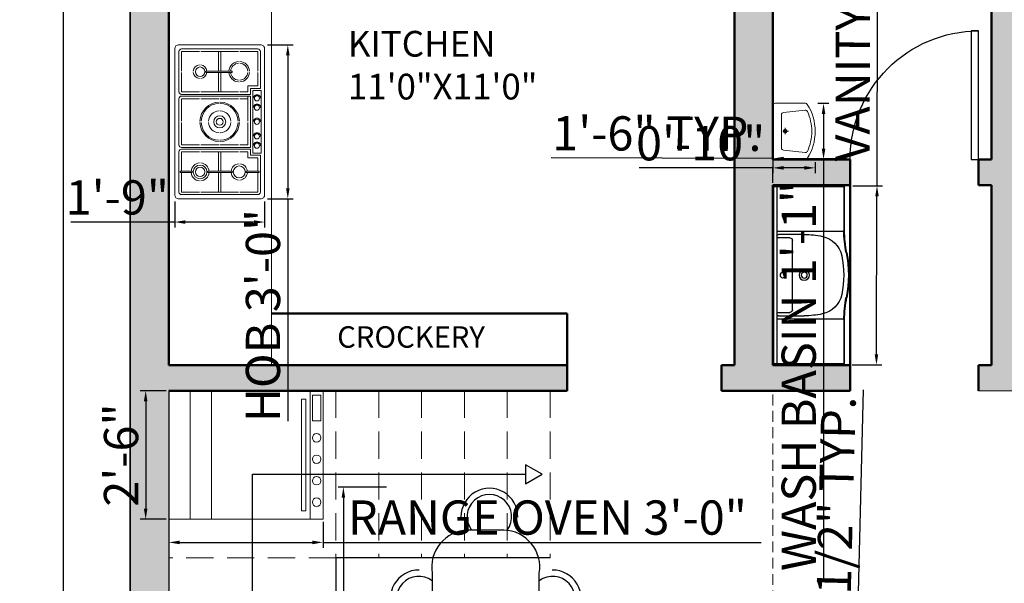
# Model space of a CAD drawing. Units: inches. Extents: x 3354 to 4308, y 1668 to 2317.
# Tile 6 of 11: x 3370 to 3600, y 2066 to 2198. Entities that reach past the tile are written whole.
import ezdxf

# ---------------------------------------------------------------- set-up
doc = ezdxf.new("R2010")
doc.units = ezdxf.units.IN
doc.linetypes.add('DASHED', pattern=[19.05, 12.7, -6.35])
for name, color, linetype, lineweight in [('A-ANNO-DIMS', 2, 'Continuous', 18), ('A-ANNO-TEXT', 7, 'Continuous', 18), ('A-AREA-IDEN', 3, 'Continuous', 18), ('A-DOOR', 3, 'Continuous', 25), ('A-EQPM', 9, 'Continuous', 18), ('A-FLOR-FIXT', 8, 'Continuous', 18), ('A-FLOR-OVHD', 8, 'DASHED', 18), ('A-FLOR-STRS', 7, 'Continuous', 25), ('A-FURN', 8, 'Continuous', 18), ('A-GLAZ', 4, 'Continuous', 18), ('A-WALL', 7, 'Continuous', 50), ('A-WALL-PATT', 8, 'Continuous', 13), ('C-PROP', 1, 'Continuous', 35)]:
    doc.layers.add(name, color=color, linetype=linetype, lineweight=lineweight)
doc.layers.add('furniture', color=7, linetype='Continuous')
doc.layers.add('SANTEH', color=7, linetype='Continuous')
doc.styles.get("Standard").update_dxf_attribs({"font": 'arial.ttf'})
doc.dimstyles.new('ISO-25', dxfattribs={"dimtxt": 8, "dimasz": 2.5, "dimexe": 1.25, "dimexo": 0.625, "dimtad": 1, "dimdec": 1, "dimlunit": 3, "dimtxsty": 'Standard', "dimcen": 2.5, "dimadec": 0, "dimazin": 0, "dimtfac": 1, "dimtdec": 1, "dimtmove": 0, "dimatfit": 3, "dimfxl": 1, "dimarcsym": 0})

# ---------------------------------------------------------------- blocks, each defined once
blk = doc.blocks.new('*U2')
for p, q in [((0, 0), (0, -6)), ((30, 0), (30, -6))]:
    blk.add_line(p, q)
blk.add_lwpolyline([(0, 0), (0, 30), (1.75, 30), (1.75, 0)], close=True)
blk.add_arc((0, 0), 30, 0, 90)
blk = doc.blocks.new('STOVE')
for p, q in [((11.85, 19.7), (11.55, 19.7)), ((11.55, 16.92), (11.55, 19.7)), ((11.85, 16.92), (11.85, 19.7)), ((11.85, 16.92), (11.55, 16.92)), ((-11.85, 13.73), (-11.85, 7.62)), ((-11.85, 13.73), (-11.55, 13.73)), ((-11.55, 13.73), (-11.55, 7.62)), ((11.85, 13.23), (11.55, 13.23)), ((11.55, 13.23), (11.55, 7.57)), ((11.85, 13.23), (11.85, 7.57)), ((-11.85, 10.75), (-16.4, 10.75)), ((-11.85, 10.25), (-16.4, 10.25)), ((-7, 10.75), (-11.55, 10.75)), ((-7, 10.25), (-11.55, 10.25)), ((7, 10.75), (11.55, 10.75)), ((7, 10.25), (11.55, 10.25)), ((11.85, 10.75), (16.4, 10.75)), ((11.85, 10.25), (16.4, 10.25)), ((-11.85, 7.62), (-11.55, 7.62)), ((11.85, 7.57), (11.55, 7.57)), ((-7, 3.9), (-8.4, 3.9)), ((-7.8, 3.3), (-7.8, 1)), ((-6.4, 3.3), (-7.8, 3.3)), ((7.3, 2.8), (-7.3, 2.8)), ((-7.3, 2.8), (-7.3, 0.8)), ((-5.4, 3.9), (-6, 3.9)), ((-5.4, 3.9), (-0.15, 3.9)), ((0.15, 3.9), (5.4, 3.9)), ((6.4, 3.3), (7.8, 3.3)), ((7, 3.9), (8.4, 3.9)), ((7.3, 2.8), (7.3, 0.8)), ((7.8, 3.3), (7.8, 1)), ((8.4, 3.9), (8.4, 1.6)), ((11.85, 4.28), (11.55, 4.28)), ((11.55, 4.28), (11.55, 1.3)), ((11.85, 4.28), (11.85, 1.3)), ((7.3, 0.8), (-7.3, 0.8)), ((11.85, 1.3), (11.55, 1.3))]:
    blk.add_line(p, q)
for points in [[(-17, 21), (17, 21, -0.414214), (18, 20), (18, 1, -0.414214), (17, 0), (-17, 0, -0.414214), (-18, 1), (-18, 20, -0.414214)], [(6, 3.3), (-6, 3.3), (-6, 19.4, -0.414214), (-5.4, 20), (5.4, 20, -0.414214), (6, 19.4)]]:
    blk.add_lwpolyline(points, format="xyb", close=True)
for points in [[(-7.8, 1), (-16.4, 1, -0.414214), (-17, 1.6), (-17, 19.4, -0.414214), (-16.4, 20), (-7, 20, -0.414214), (-6.4, 19.4), (-6.4, 3.3)], [(6.4, 19.4, -0.414214), (7, 20), (16.4, 20, -0.414214), (17, 19.4), (17, 1.6, -0.414214), (16.4, 1), (7.8, 1)]]:
    blk.add_lwpolyline(points, format="xyb")
for points in [[(-16.4, 15.22), (-16.4, 19.4), (-11.85, 19.4)], [(-11.55, 19.4), (-7, 19.4), (-7, 15.22)], [(-5.4, 15.22), (-5.4, 19.4), (-0.15, 19.4)], [(0.15, 19.4), (5.4, 19.4), (5.4, 15.22)], [(6.4, 3.3), (6.4, 19.4)], [(7, 15.22), (7, 19.4), (11.55, 19.4)], [(11.85, 19.4), (16.4, 19.4), (16.4, 15.22)], [(-16.4, 6.08), (-16.4, 14.92)], [(-7, 14.92), (-7, 6.08)], [(-5.4, 10.65), (-5.4, 14.92)], [(5.4, 14.92), (5.4, 10.65)], [(7, 6.08), (7, 14.92)], [(16.4, 14.92), (16.4, 6.08)], [(-5.4, 6.08), (-5.4, 10.35)], [(5.4, 10.35), (5.4, 6.08)], [(-11.85, 1.6), (-16.4, 1.6), (-16.4, 5.77)], [(-7, 5.77), (-7, 3.9)], [(-5.4, 3.9), (-5.4, 5.77)], [(5.4, 5.77), (5.4, 3.9)], [(7, 3.9), (7, 5.77)], [(16.4, 5.77), (16.4, 1.6), (11.85, 1.6)], [(-8.4, 3.9), (-8.4, 1.6), (-11.55, 1.6)], [(11.55, 1.6), (8.4, 1.6)]]:
    blk.add_lwpolyline(points)
for centre, radius in [((-11.7, 15.07), 1.1), ((11.7, 15.07), 1.6), ((11.7, 15.07), 1.1), ((0, 10.5), 1.4), ((0, 10.5), 0.8), ((11.7, 5.93), 1.4), ((-5.49, 1.8), 0.6), ((-3.3, 1.8), 0.6), ((0, 1.8), 0.6), ((3.39, 1.8), 0.6), ((5.57, 1.8), 0.6)]:
    blk.add_circle(centre, radius)
for centre, radius, start, end in [((-11.7, 15.07), 1.6, 95.3794, 174.6206), ((-11.7, 15.07), 1.6, 5.3794, 84.6206), ((11.7, 15.07), 2.1, 94.096, 175.904), ((11.7, 15.07), 2.1, 4.096, 85.904), ((-11.7, 15.07), 1.6, 185.3794, 264.6206), ((-11.7, 15.07), 1.6, 275.3794, 354.6206), ((0, 10.5), 4.6, 91.8687, 178.1313), ((0, 10.5), 4.3, 91.9991, 178.0009), ((0, 10.5), 4.6, 1.8687, 88.1313), ((0, 10.5), 4.3, 1.9991, 88.0009), ((11.7, 15.07), 2.1, 184.096, 265.904), ((11.7, 15.07), 2.1, 274.096, 355.904), ((0, 10.5), 2.6, 93.3074, 176.6926), ((0, 10.5), 2.6, 3.3074, 86.6926), ((0, 10.5), 4.6, 181.8687, 268.1313), ((0, 10.5), 4.3, 181.9991, 268.0009), ((0, 10.5), 2.6, 183.3074, 266.6926), ((0, 10.5), 4.6, 271.8687, 358.1313), ((0, 10.5), 4.3, 271.9991, 358.0009), ((0, 10.5), 2.6, 273.3074, 356.6926), ((-11.7, 5.93), 2.4, 93.5833, 176.4167), ((-11.7, 5.93), 2, 94.3012, 175.6988), ((-11.7, 5.93), 2.4, 3.5833, 86.4167), ((-11.7, 5.93), 2, 4.3012, 85.6988), ((11.7, 5.93), 1.9, 94.5281, 175.4719), ((11.7, 5.93), 1.9, 4.5281, 85.4719), ((-11.7, 5.93), 2.4, 183.5833, 266.4167), ((-11.7, 5.93), 2, 184.3012, 265.6988), ((-11.7, 5.93), 2.4, 273.5833, 356.4167), ((-11.7, 5.93), 2, 274.3012, 355.6988), ((11.7, 5.93), 1.9, 184.5281, 265.4719), ((11.7, 5.93), 1.9, 274.5281, 355.4719), ((-5.49, 1.8), 0.846, 89.9979, 270), ((-3.3, 1.8), 0.846, 89.9979, 270), ((0, 1.8), 0.846, 89.9979, 270), ((3.39, 1.8), 0.846, 89.9979, 270), ((5.57, 1.8), 0.846, 89.9979, 270)]:
    blk.add_arc(centre, radius, start, end)
blk = doc.blocks.new('A$C2EBB240D')
for p, q in [((0, 355.8), (0, 86.6)), ((480, 375.8), (20, 375.8)), ((500, 355.8), (500, 86.6)), ((60.8, 89.8), (82.3, 282.2)), ((250, 300), (102.1, 300)), ((250, 300), (397.9, 300)), ((439.2, 89.8), (417.7, 282.2))]:
    blk.add_line(p, q)
for points in [[(275.2, 266.4), (219.4, 266.4)], [(247.3, 238.5), (247.3, 288.9)]]:
    blk.add_lwpolyline(points)
for centre, radius, start, end in [((20, 355.8), 20, 90, 180), ((480, 355.8), 20, 0, 90), ((102.1, 280), 20, 90, 173.64284), ((247.3, 266.4), 16.7, 90, 270), ((247.3, 266.4), 10, 90, 270), ((247.3, 266.4), 16.7, 270, 90), ((247.3, 266.4), 10, 270, 90), ((397.9, 280), 20, 6.35716, 90), ((80.7, 87.6), 20, 173.64284, 244.97956), ((419.3, 87.6), 20, 295.02044, 6.35716), ((20, 86.6), 20, 180, 237.68921), ((250, 450.3), 450.3, 237.68921, 270), ((250, 450.3), 420.3, 244.97956, 270), ((250, 450.3), 450.3, 270, 302.31079), ((250, 450.3), 420.3, 270, 295.02044), ((480, 86.6), 20, 302.31079, 0)]:
    blk.add_arc(centre, radius, start, end)
blk = doc.blocks.new('s_02')
at = {"layer": 'SANTEH'}
for p, q in [((0, 0), (-519.4, -1.7)), ((0, 0), (-519.4, -1.7)), ((-520.5, -2.8), (-519.8, -209.5)), ((-520.5, -2.8), (-519.8, -209.5)), ((-517.6, -207.3), (-518.3, -5)), ((-1, -11.7), (-518.3, -13.5)), ((-517.2, -3.9), (-2.2, -2.2)), ((-387.2, -207.9), (-387.9, -13)), ((-378.3, -17.4), (-378.1, -92.6)), ((-368.3, -17.3), (-368.2, -50.3)), ((-150.9, -49.6), (-151, -16.6)), ((-140.7, -91.8), (-141, -16.6)), ((-131.4, -12.2), (-130.8, -207.1)), ((-1.1, -3.3), (-0.4, -205.6)), ((1.8, -207.7), (1.1, -1.1)), ((1.8, -207.7), (1.1, -1.1)), ((-360.4, -58.1), (-158.7, -57.4)), ((-518.7, -210.5), (-389.4, -210.1)), ((-518.7, -210.5), (-389.4, -210.1)), ((-389.4, -207.9), (-516.6, -208.4)), ((-1.5, -206.6), (-128.6, -207.1)), ((-128.6, -209.2), (0.7, -208.8)), ((-128.6, -209.2), (0.7, -208.8))]:
    blk.add_line(p, q, dxfattribs=at)
at = {"layer": 'SANTEH', "extrusion": (0, 0, -1)}
for centre, major_axis, ratio, start_param, end_param in [((0, -1.1), (-0.38, 1.02), 0.991976, 0.357514, 1.923061), ((0, -1.1), (-0.38, 1.02), 0.991976, 0.357514, 1.923061), ((-519.4, -2.8), (0, -1.09), 0.99914, 1.570796, 3.141593), ((-519.4, -2.8), (0, -1.09), 0.99914, 1.570796, 3.141593), ((-517.2, -5), (0, -1.09), 0.99914, 1.570796, 3.141593), ((-374, -17.3), (0.01, -4.35), 0.99914, 1.570796, 3.141593), ((-372.7, -17.3), (0.01, -4.35), 0.99914, 3.141593, 4.712389), ((-259.6, -29.1), (0.03, -7.61), 0.99914, 1.570796326742688, 7.853981633922275), ((-146.6, -16.6), (0.01, -4.35), 0.99914, 1.570796, 3.141593), ((-145.3, -16.6), (0.01, -4.35), 0.99914, 3.141593, 4.712389), ((-2.2, -3.3), (0, -1.09), 0.99914, 3.141593, 4.712389), ((-360.4, -50.3), (0.03, -7.83), 0.99914, 0, 1.570796), ((-158.7, -49.6), (0.03, -7.83), 0.99914, -1.570796, 0), ((-259.4, -92.2), (0.1, -15.2), 0.99914, 1.570796326791235, 7.853981633970821), ((-259.4, -92.2), (0.03, -8.7), 0.99914, 1.570796326873691, 7.853981634053277), ((-128, -91.8), (0.8, -250.2), 0.99914, 1.359365, 1.570796), ((-390.8, -92.7), (0.8, -250.2), 0.99914, -1.570796, -1.359365), ((-300.4, -129.4), (0.2, -73.7), 0.99914, 0.211723, 1.359365), ((-218.1, -129.1), (0.2, -73.7), 0.99914, -1.359365, -0.211723), ((-518.7, -209.5), (0, -1.09), 0.99914, 0, 1.570796), ((-518.7, -209.5), (0, -1.09), 0.99914, 0, 1.570796), ((-516.6, -207.3), (0, -1.09), 0.99914, 0, 1.570796), ((-388.3, -539.7), (1.1, -331.7), 0.99914, 3.141593, 3.34093), ((-388.3, -539.7), (1.1, -329.5), 0.99914, 3.141593, 3.34093), ((-388.3, -539.7), (1.1, -329.5), 0.99914, 3.141593, 3.34093), ((-260.1, 106.8), (1.1, -329.5), 0.99914, -0.199337, 0.199337), ((-260.1, 106.8), (1.1, -329.5), 0.99914, -0.199337, 0.199337), ((-260.1, 106.8), (1.1, -327.4), 0.99914, -0.199337, 0.199337), ((-259.9, 62.3), (0.9, -269.6), 0.99914, -0.211723, 0.211723), ((-127.5, -538.8), (1.1, -331.7), 0.99914, 2.942255, 3.141593), ((-127.5, -538.8), (1.1, -329.5), 0.99914, 2.942255, 3.141593), ((-127.5, -538.8), (1.1, -329.5), 0.99914, 2.942255, 3.141593), ((-1.5, -205.6), (0, -1.09), 0.99914, 4.712389, 6.283185), ((0.7, -207.7), (0, -1.09), 0.99914, 4.712389, 6.283185), ((0.7, -207.7), (0, -1.09), 0.99914, 4.712389, 6.283185)]:
    blk.add_ellipse(centre, major_axis=major_axis, ratio=ratio, start_param=start_param, end_param=end_param, dxfattribs=at)
blk = doc.blocks.new('Range-Oven - 30 in front')
for p, q in [((0, 33.00005), (30, 33.00005)), ((30, 10), (0, 10)), ((0, 5), (30, 5))]:
    blk.add_line(p, q)
for points in [[(0, 0), (0, 36.00005), (30, 36.00005), (30, 0)], [(1, 33.50005), (1, 35.50005), (7, 35.50005), (7, 33.50005)], [(2, 31.00005), (2, 32.00005), (28, 32.00005), (28, 31.00005)]]:
    blk.add_lwpolyline(points, close=True)
for centre in [(11, 34.50005), (16, 34.50005), (21, 34.50005), (26, 34.50005)]:
    blk.add_circle(centre, 1)
blk = doc.blocks.new('DINING')
at = {"layer": 'furniture'}
for p, q in [((67.79, 20.83), (16.8, 20.83)), ((0, 7.03), (0, -7.03)), ((84.59, -7.03), (84.59, 7.03)), ((16.8, -20.83), (67.79, -20.83))]:
    blk.add_line(p, q, dxfattribs=at)
for centre, radius, start, end in [((26.6, 26.01), 11.04, 359.2862, 180.7138), ((26.6, 26.01), 8.64, 323.1301, 216.8699), ((59.5, 26.01), 11.04, 359.2862, 180.7138), ((59.5, 26.01), 8.64, 318.7837, 216.8699), ((14.46, 6.55), 14.47, 80.6926, 178.1087), ((70.13, 6.55), 14.47, 1.8913, 99.3074), ((-5.19, 1.43), 11.04, 89.2862, 270.7138), ((90.13, 1.43), 11.04, 269.2862, 90.7138), ((-5.19, 1.43), 8.64, 53.1301, 306.8699), ((90.13, 1.43), 8.64, 233.1301, 126.8699), ((14.46, -6.55), 14.47, 181.8913, 279.3074), ((70.13, -6.55), 14.47, 260.6926, 358.1087), ((26.6, -26.01), 8.64, 143.1301, 36.8699), ((59.5, -26.01), 8.64, 143.1301, 41.2163), ((26.6, -26.01), 11.04, 179.2862, 0.7138), ((59.5, -26.01), 11.04, 179.2862, 0.7138)]:
    blk.add_arc(centre, radius, start, end, dxfattribs=at)
blk = doc.blocks.new('*D50')
at = {"layer": 'A-ANNO-DIMS', "color": 0, "lineweight": -2, "transparency": 16777216}
for p, q in [((3395.65, 2294.3), (3379.37, 2294.3)), ((3380.62, 2291.8), (3380.62, 1756.8)), ((3395.65, 1754.3), (3379.37, 1754.3))]:
    blk.add_line(p, q, dxfattribs=at)
at = {"layer": 'A-ANNO-DIMS', "color": 0, "transparency": 16777216}
for points in [[(3380.2, 2291.8), (3381.04, 2291.8), (3380.62, 2294.3)], [(3380.2, 1756.8), (3381.04, 1756.8), (3380.62, 1754.3)]]:
    blk.add_solid(points, dxfattribs=at)
at = {"layer": 'Defpoints', "color": 0, "transparency": 16777216}
for p in [(3396.28, 2294.3), (3380.62, 1754.3), (3396.28, 1754.3)]:
    blk.add_point(p, dxfattribs=at)
at = {"layer": 'A-ANNO-DIMS', "color": 0, "transparency": 16777216, "insert": (3375.93, 2024.3), "char_height": 8, "attachment_point": 5, "rotation": 90}
blk.add_mtext("45'", dxfattribs=at)
blk = doc.blocks.new('*D66')
at = {"layer": 'A-ANNO-DIMS', "color": 0, "lineweight": -2, "transparency": 16777216}
for p, q in [((3565.2, 2022.8), (3567.45, 2111.51)), ((3560.34, 2022.92), (3566.45, 2022.77)), ((3564.33, 1988.78), (3565.13, 2020.3)), ((3559.42, 1986.4), (3565.52, 1986.25))]:
    blk.add_line(p, q, dxfattribs=at)
at = {"layer": 'A-ANNO-DIMS', "color": 0, "transparency": 16777216}
for points in [[(3564.72, 2020.31), (3565.55, 2020.29), (3565.2, 2022.8)], [(3563.92, 1988.79), (3564.75, 1988.77), (3564.27, 1986.28)]]:
    blk.add_solid(points, dxfattribs=at)
at = {"layer": 'Defpoints', "color": 0, "transparency": 16777216}
for p in [(3559.72, 2022.94), (3565.2, 2022.8), (3558.79, 1986.42)]:
    blk.add_point(p, dxfattribs=at)
at = {"layer": 'A-ANNO-DIMS', "color": 0, "transparency": 16777216, "insert": (3561.6, 2068.53), "char_height": 8, "attachment_point": 5, "rotation": 88.5431}
blk.add_mtext('TV 3\'-0 1/2" TYP.', dxfattribs=at)
blk = doc.blocks.new('*D68')
at = {"layer": 'A-ANNO-DIMS', "color": 0, "lineweight": -2, "transparency": 16777216}
for p, q in [((3570.57, 2159.15), (3570.89, 2255.55)), ((3564.92, 2159.17), (3571.82, 2159.15)), ((3570.44, 2119.83), (3570.56, 2156.65)), ((3564.78, 2117.35), (3571.68, 2117.33))]:
    blk.add_line(p, q, dxfattribs=at)
at = {"layer": 'A-ANNO-DIMS', "color": 0, "transparency": 16777216}
for points in [[(3570.14, 2156.65), (3570.98, 2156.65), (3570.57, 2159.15)], [(3570.02, 2119.83), (3570.85, 2119.83), (3570.43, 2117.33)]]:
    blk.add_solid(points, dxfattribs=at)
at = {"layer": 'Defpoints', "color": 0, "transparency": 16777216}
for p in [(3564.29, 2159.17), (3570.57, 2159.15), (3564.15, 2117.35)]:
    blk.add_point(p, dxfattribs=at)
at = {"layer": 'A-ANNO-DIMS', "color": 0, "transparency": 16777216, "insert": (3566.02, 2208.62), "char_height": 8, "attachment_point": 5, "rotation": 89.8084}
blk.add_mtext('VANITY 3\'-6" TYP.', dxfattribs=at)
blk = doc.blocks.new('*D69')
at = {"layer": 'A-ANNO-DIMS', "color": 0, "lineweight": -2, "transparency": 16777216}
for p, q in [((3546.3, 2165.51), (3494.54, 2165.68)), ((3546.28, 2159.86), (3546.3, 2166.76)), ((3561.81, 2165.45), (3548.8, 2165.5)), ((3564.3, 2159.8), (3564.32, 2166.7))]:
    blk.add_line(p, q, dxfattribs=at)
at = {"layer": 'A-ANNO-DIMS', "color": 0, "transparency": 16777216}
for points in [[(3548.8, 2165.92), (3548.8, 2165.08), (3546.3, 2165.51)], [(3561.82, 2165.87), (3561.81, 2165.04), (3564.31, 2165.45)]]:
    blk.add_solid(points, dxfattribs=at)
at = {"layer": 'Defpoints', "color": 0, "transparency": 16777216}
for p in [(3546.3, 2165.51), (3546.28, 2159.23), (3564.29, 2159.17)]:
    blk.add_point(p, dxfattribs=at)
at = {"layer": 'A-ANNO-DIMS', "color": 0, "transparency": 16777216, "insert": (3519.18, 2170.31), "char_height": 8, "attachment_point": 5, "rotation": 359.8084}
blk.add_mtext('1\'-6" TYP.', dxfattribs=at)
blk = doc.blocks.new('*D78')
at = {"layer": 'A-ANNO-DIMS', "color": 0, "lineweight": -2, "transparency": 16777216}
for p, q in [((3428.28, 2192.08), (3434.3, 2192.08)), ((3433.05, 2189.58), (3433.05, 2158.58)), ((3428.28, 2156.08), (3434.3, 2156.08)), ((3433.05, 2156.08), (3433.05, 2104.17))]:
    blk.add_line(p, q, dxfattribs=at)
at = {"layer": 'A-ANNO-DIMS', "color": 0, "transparency": 16777216}
for points in [[(3432.64, 2189.58), (3433.47, 2189.58), (3433.05, 2192.08)], [(3432.64, 2158.58), (3433.47, 2158.58), (3433.05, 2156.08)]]:
    blk.add_solid(points, dxfattribs=at)
at = {"layer": 'Defpoints', "color": 0, "transparency": 16777216}
for p in [(3427.65, 2192.08), (3427.65, 2156.08), (3433.05, 2156.08)]:
    blk.add_point(p, dxfattribs=at)
at = {"layer": 'A-ANNO-DIMS', "color": 0, "transparency": 16777216, "insert": (3428.29, 2128.87), "char_height": 8, "attachment_point": 5, "rotation": 90}
blk.add_mtext('HOB 3\'-0"', dxfattribs=at)
blk = doc.blocks.new('*D79')
at = {"layer": 'A-ANNO-DIMS', "color": 0, "lineweight": -2, "transparency": 16777216}
for p, q in [((3406.65, 2155.45), (3406.65, 2149.43)), ((3427.65, 2155.45), (3427.65, 2149.43)), ((3406.65, 2150.68), (3382.39, 2150.68)), ((3425.15, 2150.68), (3409.15, 2150.68))]:
    blk.add_line(p, q, dxfattribs=at)
at = {"layer": 'A-ANNO-DIMS', "color": 0, "transparency": 16777216}
for points in [[(3409.15, 2151.09), (3409.15, 2150.26), (3406.65, 2150.68)], [(3425.15, 2151.09), (3425.15, 2150.26), (3427.65, 2150.68)]]:
    blk.add_solid(points, dxfattribs=at)
at = {"layer": 'Defpoints', "color": 0, "transparency": 16777216}
for p in [(3406.65, 2156.08), (3427.65, 2156.08), (3406.65, 2150.68)]:
    blk.add_point(p, dxfattribs=at)
at = {"layer": 'A-ANNO-DIMS', "color": 0, "transparency": 16777216, "insert": (3393.27, 2155.39), "char_height": 8, "attachment_point": 5}
blk.add_mtext('1\'-9"', dxfattribs=at)
blk = doc.blocks.new('*D82')
at = {"layer": 'A-ANNO-DIMS', "color": 0, "lineweight": -2, "transparency": 16777216}
for p, q in [((3556.75, 2178.4), (3559.34, 2178.4)), ((3558.09, 2175.9), (3558.09, 2167.8)), ((3556.75, 2165.3), (3559.34, 2165.3)), ((3558.09, 2165.3), (3558.09, 2066.68))]:
    blk.add_line(p, q, dxfattribs=at)
at = {"layer": 'A-ANNO-DIMS', "color": 0, "transparency": 16777216}
for points in [[(3557.68, 2175.9), (3558.51, 2175.9), (3558.09, 2178.4)], [(3557.68, 2167.8), (3558.51, 2167.8), (3558.09, 2165.3)]]:
    blk.add_solid(points, dxfattribs=at)
at = {"layer": 'Defpoints', "color": 0, "transparency": 16777216}
for p in [(3556.13, 2178.4), (3556.13, 2165.3), (3558.09, 2165.3)]:
    blk.add_point(p, dxfattribs=at)
at = {"layer": 'A-ANNO-DIMS', "color": 0, "transparency": 16777216, "insert": (3553.33, 2114.74), "char_height": 8, "attachment_point": 5, "rotation": 90}
blk.add_mtext('WASH BASIN 1\'-1"', dxfattribs=at)
blk = doc.blocks.new('*D83')
at = {"layer": 'A-ANNO-DIMS', "color": 0, "lineweight": -2, "transparency": 16777216}
for p, q in [((3546.28, 2163.33), (3515.05, 2163.33)), ((3546.28, 2164.67), (3546.28, 2162.08)), ((3553.63, 2163.33), (3548.78, 2163.33)), ((3556.13, 2164.67), (3556.13, 2162.08))]:
    blk.add_line(p, q, dxfattribs=at)
at = {"layer": 'A-ANNO-DIMS', "color": 0, "transparency": 16777216}
for points in [[(3548.78, 2163.75), (3548.78, 2162.91), (3546.28, 2163.33)], [(3553.63, 2163.75), (3553.63, 2162.91), (3556.13, 2163.33)]]:
    blk.add_solid(points, dxfattribs=at)
at = {"layer": 'Defpoints', "color": 0, "transparency": 16777216}
for p in [(3546.28, 2165.3), (3556.13, 2165.3), (3546.28, 2163.33)]:
    blk.add_point(p, dxfattribs=at)
at = {"layer": 'A-ANNO-DIMS', "color": 0, "transparency": 16777216, "insert": (3529.41, 2168.04), "char_height": 8, "attachment_point": 5}
blk.add_mtext('0\'-10"', dxfattribs=at)
blk = doc.blocks.new('*D88')
at = {"layer": 'A-ANNO-DIMS', "color": 0, "lineweight": -2, "transparency": 16777216}
for p, q in [((3405.28, 2080.67), (3405.28, 2074.65)), ((3441.28, 2080.67), (3441.28, 2074.65)), ((3407.78, 2075.9), (3438.78, 2075.9)), ((3441.28, 2075.9), (3543.5, 2075.9))]:
    blk.add_line(p, q, dxfattribs=at)
at = {"layer": 'A-ANNO-DIMS', "color": 0, "transparency": 16777216}
for points in [[(3407.78, 2076.31), (3407.78, 2075.48), (3405.28, 2075.9)], [(3438.78, 2076.31), (3438.78, 2075.48), (3441.28, 2075.9)]]:
    blk.add_solid(points, dxfattribs=at)
at = {"layer": 'Defpoints', "color": 0, "transparency": 16777216}
for p in [(3405.28, 2081.3), (3441.28, 2081.3), (3441.28, 2075.9)]:
    blk.add_point(p, dxfattribs=at)
at = {"layer": 'A-ANNO-DIMS', "color": 0, "transparency": 16777216, "insert": (3493.64, 2080.66), "char_height": 8, "attachment_point": 5}
blk.add_mtext('RANGE OVEN 3\'-0"', dxfattribs=at)
blk = doc.blocks.new('*D89')
at = {"layer": 'A-ANNO-DIMS', "color": 0, "lineweight": -2, "transparency": 16777216}
for p, q in [((3404.65, 2111.3), (3398.63, 2111.3)), ((3399.88, 2108.8), (3399.88, 2083.8)), ((3404.65, 2081.3), (3398.63, 2081.3))]:
    blk.add_line(p, q, dxfattribs=at)
at = {"layer": 'A-ANNO-DIMS', "color": 0, "transparency": 16777216}
for points in [[(3399.46, 2108.8), (3400.29, 2108.8), (3399.88, 2111.3)], [(3399.46, 2083.8), (3400.29, 2083.8), (3399.88, 2081.3)]]:
    blk.add_solid(points, dxfattribs=at)
at = {"layer": 'Defpoints', "color": 0, "transparency": 16777216}
for p in [(3405.28, 2111.3), (3399.88, 2081.3), (3405.28, 2081.3)]:
    blk.add_point(p, dxfattribs=at)
at = {"layer": 'A-ANNO-DIMS', "color": 0, "transparency": 16777216, "insert": (3395.17, 2096.3), "char_height": 8, "attachment_point": 5, "rotation": 90}
blk.add_mtext('2\'-6"', dxfattribs=at)
blk = doc.blocks.new('*D90')
at = {"layer": 'A-ANNO-DIMS', "color": 0, "lineweight": -2, "transparency": 16777216}
for p, q in [((3456.06, 2088.83), (3444.77, 2088.83)), ((3446.02, 2086.33), (3446.02, 2020.22)), ((3456.06, 2017.72), (3444.77, 2017.72)), ((3446.02, 2017.72), (3446.02, 1919.83))]:
    blk.add_line(p, q, dxfattribs=at)
at = {"layer": 'A-ANNO-DIMS', "color": 0, "transparency": 16777216}
for points in [[(3445.6, 2086.33), (3446.44, 2086.33), (3446.02, 2088.83)], [(3445.6, 2020.22), (3446.44, 2020.22), (3446.02, 2017.72)]]:
    blk.add_solid(points, dxfattribs=at)
at = {"layer": 'Defpoints', "color": 0, "transparency": 16777216}
for p in [(3456.69, 2088.83), (3446.02, 2017.72), (3456.69, 2017.72)]:
    blk.add_point(p, dxfattribs=at)
at = {"layer": 'A-ANNO-DIMS', "color": 0, "transparency": 16777216, "insert": (3441.26, 1967.53), "char_height": 8, "attachment_point": 5, "rotation": 90}
blk.add_mtext('DINING SET 5\'-11"', dxfattribs=at)

msp = doc.modelspace()

# ---------------------------------------------------------------- hatches: boundary and pattern name
at = {"layer": 'A-WALL-PATT', "transparency": 33554687}
h = msp.add_hatch(color=256, dxfattribs=at)
h.dxf.hatch_style = 1
h.paths.add_polyline_path([(3546.28, 1829.3), (3552.28, 1829.3), (3552.28, 1838.3), (3546.28, 1838.3), (3546.28, 1910.3), (3582.28, 1910.3), (3582.28, 1919.3), (3546.28, 1919.3), (3546.28, 1961.3), (3534.28, 1961.3), (3534.28, 1955.3), (3537.28, 1955.3), (3537.28, 1808.3), (3516.28, 1808.3), (3516.28, 1799.3), (3546.28, 1799.3)])
h.paths.add_polyline_path([(3672.28, 1919.3), (3656.51, 1919.3), (3630.28, 1919.3), (3630.28, 1910.3), (3642.28, 1910.3), (3642.28, 1838.3), (3630.28, 1838.3), (3630.28, 1835.3), (3630.28, 1829.3), (3642.28, 1829.3), (3642.28, 1799.3), (3651.28, 1799.3), (3651.28, 1910.3), (3672.28, 1910.3)])
h.paths.add_polyline_path([(3744.28, 1959.8), (3735.28, 1959.8), (3735.28, 1923.23), (3735.28, 1919.3), (3714.28, 1919.3), (3714.28, 1910.3), (3744.28, 1910.3)])
h.paths.add_polyline_path([(3744.28, 2072.3), (3735.28, 2072.3), (3735.28, 2031.8), (3744.28, 2031.8)])
h.paths.add_polyline_path([(3744.28, 2150.3), (3735.28, 2150.3), (3735.28, 2108.3), (3744.28, 2108.3)])
h.paths.add_polyline_path([(3744.28, 2258.3), (3705.28, 2258.3), (3705.28, 2249.3), (3735.28, 2249.3), (3735.28, 2210.3), (3744.28, 2210.3)])
h.paths.add_polyline_path([(3633.28, 2258.3), (3583.78, 2258.3), (3583.78, 2249.3), (3588.24, 2249.3), (3597.28, 2249.3), (3597.28, 2165.3), (3594.28, 2165.3), (3594.28, 2159.3), (3597.28, 2159.3), (3597.28, 2117.3), (3594.28, 2117.3), (3594.28, 2111.3), (3603.28, 2111.3), (3603.28, 2249.3), (3633.28, 2249.3)])
h.paths.add_polyline_path([(3559.78, 2258.3), (3492.28, 2258.3), (3492.28, 2249.3), (3537.28, 2249.3), (3537.28, 2117.3), (3534.28, 2117.3), (3534.28, 2111.3), (3564.28, 2111.3), (3564.28, 2117.3), (3546.28, 2117.3), (3546.28, 2159.3), (3564.28, 2159.3), (3564.28, 2165.3), (3546.28, 2165.3), (3546.28, 2249.3), (3559.78, 2249.3)])
h.paths.add_polyline_path([(3450.28, 2258.3), (3396.28, 2258.3), (3396.28, 1799.3), (3474.28, 1799.3), (3474.28, 1808.3), (3405.28, 1808.3), (3405.28, 1955.3), (3498.28, 1955.3), (3498.28, 1961.3), (3405.28, 1961.3), (3405.28, 2111.3), (3498.28, 2111.3), (3498.28, 2117.3), (3405.28, 2117.3), (3405.28, 2249.3), (3450.28, 2249.3)])
h.paths.add_polyline_path([(3582.28, 1838.3), (3576.28, 1838.3), (3576.28, 1829.3), (3582.28, 1829.3)], flags=17)

# ---------------------------------------------------------------- linework, layer by layer
at = {"layer": 'A-FLOR-OVHD', "ltscale": 0.5}
for p, q in [((3444.28, 2111.3), (3444.28, 2072.3)), ((3454.28, 2111.3), (3454.28, 2072.3)), ((3464.28, 2111.3), (3464.28, 2072.3)), ((3474.28, 2111.3), (3474.28, 2072.3)), ((3484.28, 2111.3), (3484.28, 2072.3)), ((3494.28, 2111.3), (3494.28, 2072.3)), ((3444.28, 2072.3), (3405.28, 2072.3))]:
    msp.add_line(p, q, dxfattribs=at)
at = {"layer": 'A-FLOR-OVHD', "ltscale": 0.2}
msp.add_line((3546.28, 2039.3), (3546.28, 2111.3), dxfattribs=at)
at = {"layer": 'A-FLOR-STRS'}
for p, q in [((3405.28, 2111.3), (3405.28, 1961.3)), ((3444.28, 2072.3), (3444.28, 1961.3)), ((3494.28, 2072.3), (3444.28, 2072.3))]:
    msp.add_line(p, q, dxfattribs=at)
msp.add_lwpolyline([(3492.43, 2091.8), (3488.54, 2094.04), (3488.54, 2089.55)], close=True, dxfattribs=at)
msp.add_lwpolyline([(3494.28, 1980.8), (3424.78, 1980.8), (3424.78, 2091.8), (3488.54, 2091.8)], dxfattribs=at)
at = {"layer": 'A-FURN'}
msp.add_line((3429.28, 2225.3), (3429.28, 2117.3), dxfattribs=at)
at = {"layer": 'A-GLAZ'}
msp.add_line((3603.28, 2111.3), (3594.28, 2111.3), dxfattribs=at)
at = {"layer": 'A-WALL'}
for p, q in [((3405.28, 2249.3), (3405.28, 2117.3)), ((3537.28, 2249.3), (3537.28, 2117.3)), ((3546.28, 2249.3), (3546.28, 2165.3)), ((3597.28, 2165.3), (3597.28, 2249.3)), ((3564.28, 2165.3), (3546.28, 2165.3)), ((3564.28, 2117.3), (3564.28, 2165.3)), ((3597.28, 2165.3), (3594.28, 2165.3)), ((3594.28, 2159.3), (3594.28, 2165.3)), ((3546.28, 2159.3), (3546.28, 2117.3)), ((3564.28, 2159.3), (3546.28, 2159.3)), ((3597.28, 2159.3), (3594.28, 2159.3)), ((3597.28, 2117.3), (3597.28, 2159.3)), ((3498.28, 2129.3), (3429.28, 2129.3)), ((3498.28, 2129.3), (3498.28, 2111.3)), ((3498.28, 2117.3), (3405.28, 2117.3)), ((3534.28, 2117.3), (3534.28, 2111.3)), ((3537.28, 2117.3), (3534.28, 2117.3)), ((3564.28, 2117.3), (3546.28, 2117.3)), ((3564.28, 2111.3), (3564.28, 2117.3)), ((3597.28, 2117.3), (3594.28, 2117.3)), ((3594.28, 2111.3), (3594.28, 2117.3)), ((3498.28, 2111.3), (3405.28, 2111.3)), ((3564.28, 2111.3), (3534.28, 2111.3))]:
    msp.add_line(p, q, dxfattribs=at)
at = {"layer": 'C-PROP'}
msp.add_lwpolyline([(3738.28, 1754.3), (3780.28, 1754.3), (3780.28, 2294.3), (3396.28, 2294.3), (3396.28, 1754.3), (3576.28, 1754.3)], dxfattribs=at)

# ---------------------------------------------------------------- block references
at = {"layer": 'A-DOOR', "xscale": -1}
msp.add_blockref('*U2', (3594.28, 2165.3), dxfattribs=at)
at = {"layer": 'A-EQPM', "xscale": -1, "rotation": 90}
msp.add_blockref('STOVE', (3427.65, 2174.08), dxfattribs=at)
at = {"layer": 'A-EQPM', "rotation": 270}
msp.add_blockref('Range-Oven - 30 in front', (3405.28, 2111.3), dxfattribs=at)
at = {"layer": 'A-FLOR-FIXT'}
for name, p, xscale, yscale, zscale, rotation in [('A$C2EBB240D', (3556.13, 2178.4), -0.026211548048557, 0.026211548048557, 0.026211548048557, 90), ('s_02', (3546.28, 2159.09), 0.0800758531328607, 0.0800758531328607, 0.0800758531328607, 89.80836855164229)]:
    msp.add_blockref(name, p, dxfattribs=dict(at, xscale=xscale, yscale=yscale, zscale=zscale, rotation=rotation))
at = {"layer": 'A-FURN', "xscale": 0.6005281001188298, "yscale": 0.6005281001188298, "zscale": 0.6005281001188298, "rotation": 270}
msp.add_blockref('DINING', (3479.24, 2078.78), dxfattribs=at)

# ---------------------------------------------------------------- texts
at = {"layer": 'A-ANNO-TEXT', "insert": (3444.58, 2126.35), "char_height": 5, "attachment_point": 1}
msp.add_mtext_dynamic_manual_height_columns('CROCKERY', width=74.5832, gutter_width=12.5, heights=[0], dxfattribs=at)
at = {"layer": 'A-AREA-IDEN', "insert": (3447.05, 2195.3), "char_height": 6, "attachment_point": 1}
msp.add_mtext_dynamic_manual_height_columns('KITCHEN\\P11\'0"X11\'0"', width=74.5832, gutter_width=12.5, heights=[0], dxfattribs=at)

# ---------------------------------------------------------------- dimensions: what is measured, and where the dimension line sits
at = {"layer": 'A-ANNO-DIMS'}
for base, p1, p2, angle, override, picture, middle in [((3380.62, 1754.3), (3396.28, 2294.3), (3396.28, 1754.3), 90, {"dimclrd": 0, "dimclre": 0, "dimclrt": 0}, '*D50', (3375.93, 2024.3)), ((3546.2768, 2163.3306), (3556.1265, 2165.2965), (3546.2768, 2165.2965), 180, {"dimdec": 1, "dimrnd": 0, "dimzin": 1, "dimlunit": 4, "dimfrac": 2}, '*D83', (3529.4111, 2168.0402)), ((3406.65, 2150.68), (3427.65, 2156.08), (3406.65, 2156.08), 180, {"dimdec": 1, "dimrnd": 0, "dimzin": 1, "dimlunit": 4, "dimfrac": 2}, '*D79', (3393.27, 2155.39)), ((3399.88, 2081.3), (3405.28, 2111.3), (3405.28, 2081.3), 270, {"dimdec": 1, "dimrnd": 0, "dimzin": 1, "dimlunit": 4, "dimfrac": 2}, '*D89', (3395.17, 2096.3))]:
    dim = msp.add_linear_dim(base=base, p1=p1, p2=p2, angle=angle, dimstyle='ISO-25', override=override, dxfattribs=at)
    dim.commit()
    dim.dimension.update_dxf_attribs({"geometry": picture, "text_midpoint": middle})
for base, p1, p2, angle, text, picture, middle in [((3570.57, 2159.15), (3564.15, 2117.35), (3564.29, 2159.17), 89.8084, 'VANITY <> TYP.', '*D68', (3566.02, 2208.62)), ((3433.05, 2156.08), (3427.65, 2192.08), (3427.65, 2156.08), 270, 'HOB <>', '*D78', (3428.29, 2128.87)), ((3546.3, 2165.51), (3564.29, 2159.17), (3546.28, 2159.23), 179.8084, '<> TYP.', '*D69', (3519.18, 2170.31)), ((3558.09, 2165.3), (3556.13, 2178.4), (3556.13, 2165.3), 270, 'WASH BASIN <>', '*D82', (3553.33, 2114.74)), ((3565.2, 2022.8), (3558.79, 1986.42), (3559.72, 2022.94), 88.5431, 'TV <> TYP.', '*D66', (3561.6, 2068.53)), ((3446.02, 2017.72), (3456.69, 2088.83), (3456.69, 2017.72), 270, 'DINING SET <>', '*D90', (3441.26, 1967.53))]:
    dim = msp.add_linear_dim(base=base, p1=p1, p2=p2, angle=angle, text=text, dimstyle='ISO-25', override={"dimdec": 1, "dimrnd": 0, "dimzin": 1, "dimlunit": 4, "dimfrac": 2}, dxfattribs=at)
    dim.commit()
    dim.dimension.update_dxf_attribs({"geometry": picture, "text_midpoint": middle})
dim = msp.add_linear_dim(base=(3441.28, 2075.9), p1=(3405.28, 2081.3), p2=(3441.28, 2081.3), text='RANGE OVEN <>', dimstyle='ISO-25', override={"dimdec": 1, "dimrnd": 0, "dimzin": 1, "dimlunit": 4, "dimfrac": 2}, dxfattribs=at)
dim.commit()
dim.dimension.update_dxf_attribs({"geometry": '*D88', "text_midpoint": (3493.64, 2080.66)})

doc.saveas('drawing.dxf')
